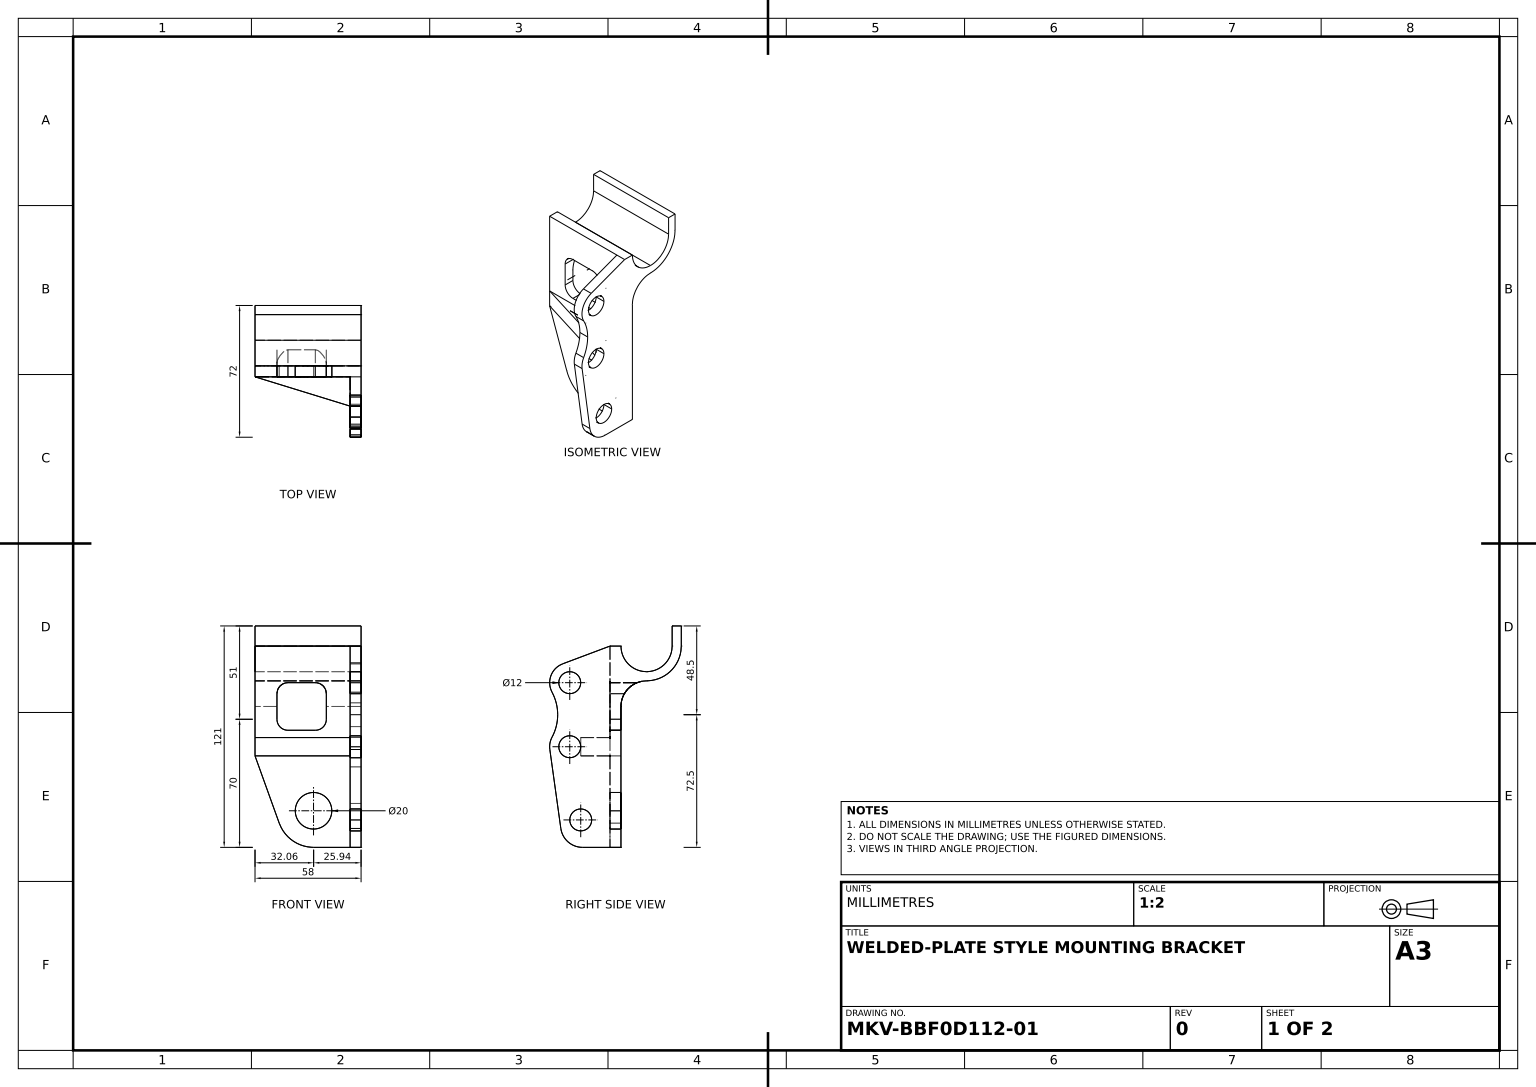
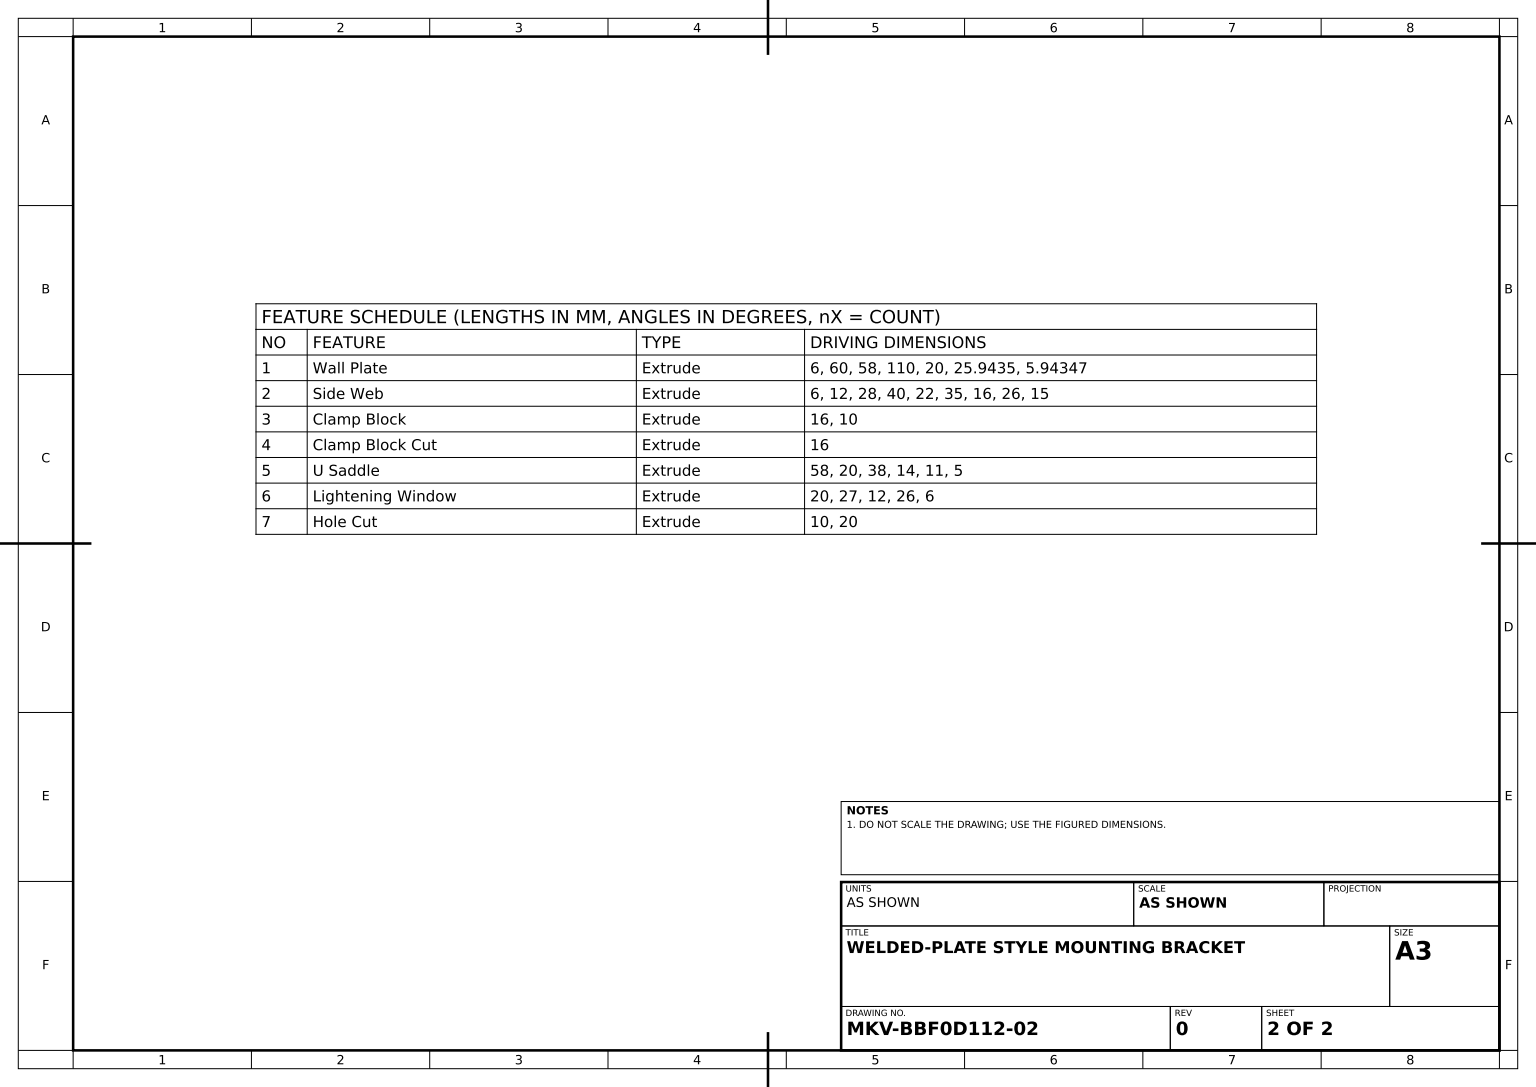
from build123d import *

# Parameters (mm, degrees)
WALL_PLATE_DEPTH           = 6
SIDE_WEB_SKETCH_R          = 6
SIDE_WEB_DEPTH             = 6
CLAMP_BLOCK_SKETCH_W       = 52
CLAMP_BLOCK_SKETCH_H       = 10
CLAMP_BLOCK_DEPTH          = 16
CLAMP_BLOCK_CUT_DEPTH      = 93.11405973
CLAMP_BLOCK_CUT_DEPTH_BACK = 16
U_SADDLE_DEPTH             = 58
LIGHTENING_WINDOW_DEPTH    = 20
HOLE_SKETCH_R              = 10
HOLE_CUT_DEPTH             = 10


with BuildPart() as part:
    # Wall Plate Sketch → Wall Plate (new body)
    with BuildSketch(Plane.XY):
        with BuildLine():
            Line((0, 0), (0, -60))
            Line((0, -60), (13.238780172, -96.774389365))
            ThreePointArc((13.238780172, -96.774389365), (20.556262919, -106.362881582), (32.056528409, -110))
            Line((32.056528409, -110), (38, -110))
            Line((38, -110), (58, -110))
            Line((58, -110), (58, 0))
            Line((58, 0), (0, 0))
        make_face()
    extrude(amount=WALL_PLATE_DEPTH)

    # Side Web Sketch → Side Web (add)
    with BuildSketch(Plane(origin=(58, 0, 0), x_dir=(0, 0, -1), z_dir=(1, 0, 0))):
        with BuildLine():
            ThreePointArc((-21, -110), (-28.878172083, -107.051762515), (-32.885223791, -99.655734106))
            Line((-32.885223791, -99.655734106), (-38.894788475, -56.517756263))
            ThreePointArc((-38.894788475, -56.517756263), (-38.82790492, -53.0618372), (-37.691846294, -49.797297297))
            ThreePointArc((-37.691846294, -49.797297297), (-34.599846625, -37.5), (-37.691846294, -25.202702703))
            ThreePointArc((-37.691846294, -25.202702703), (-38.296228327, -16.128607197), (-31.863054321, -9.700640247))
            Line((-31.863054321, -9.700640247), (-6, 0))
            Line((-6, 0), (-6, -110))
            Line((-6, -110), (-21, -110))
        make_face()
        with Locations((-22, -95)):
            Circle(SIDE_WEB_SKETCH_R, mode=Mode.SUBTRACT)
        with Locations((-28, -55)):
            Circle(SIDE_WEB_SKETCH_R, mode=Mode.SUBTRACT)
        with Locations((-28, -20)):
            Circle(SIDE_WEB_SKETCH_R, mode=Mode.SUBTRACT)
    extrude(amount=-SIDE_WEB_DEPTH)

    # Clamp Block Sketch → Clamp Block (add)
    with BuildSketch(Plane.XY.offset(6)):
        with Locations((26, -55)):
            Rectangle(CLAMP_BLOCK_SKETCH_W, CLAMP_BLOCK_SKETCH_H)
    extrude(amount=CLAMP_BLOCK_DEPTH)

    # Clamp Block Cut Sketch → Clamp Block Cut (cut, two sides: drawn at the far end of the back side and taken through both)
    with BuildSketch(Plane(origin=(0, -50, 0), x_dir=(1, 0, 0), z_dir=(0, 1, 0)).offset(-CLAMP_BLOCK_CUT_DEPTH_BACK)):
        Polygon((0, -22), (52, -22), (0, -6), align=None)
    extrude(amount=CLAMP_BLOCK_CUT_DEPTH + CLAMP_BLOCK_CUT_DEPTH_BACK, mode=Mode.SUBTRACT)

    # U Saddle Sketch → U Saddle (add)
    with BuildSketch(Plane.ZY):
        with BuildLine():
            Line((0, -33), (0, 0))
            ThreePointArc((0, 0), (-14, -14), (-28, 0))
            Line((-28, 0), (-28, 11))
            Line((-28, 11), (-33, 11))
            Line((-33, 11), (-33, 0))
            ThreePointArc((-33, 0), (-27.435028843, -13.435028843), (-14, -19))
            ThreePointArc((-14, -19), (-4.100505063, -23.100505063), (0, -33))
        make_face()
    extrude(amount=-U_SADDLE_DEPTH)

    # Lightening Window Sketch → Lightening Window (cut)
    with BuildSketch(Plane.XY.offset(6)):
        with BuildLine():
            Line((18, -20), (33, -20))
            ThreePointArc((33, -20), (37.242640687, -21.757359313), (39, -26))
            Line((39, -26), (39, -40))
            ThreePointArc((39, -40), (37.242640687, -44.242640687), (33, -46))
            Line((33, -46), (18, -46))
            ThreePointArc((18, -46), (13.757359313, -44.242640687), (12, -40))
            Line((12, -40), (12, -26))
            ThreePointArc((12, -26), (13.757359313, -21.757359313), (18, -20))
        make_face()
    extrude(amount=-LIGHTENING_WINDOW_DEPTH, mode=Mode.SUBTRACT)

    # Hole Sketch → Hole Cut (cut)
    with BuildSketch(Plane.XY.offset(6)):
        with Locations((32, -90)):
            Circle(HOLE_SKETCH_R)
    extrude(amount=-HOLE_CUT_DEPTH, mode=Mode.SUBTRACT)


solid = part.part
